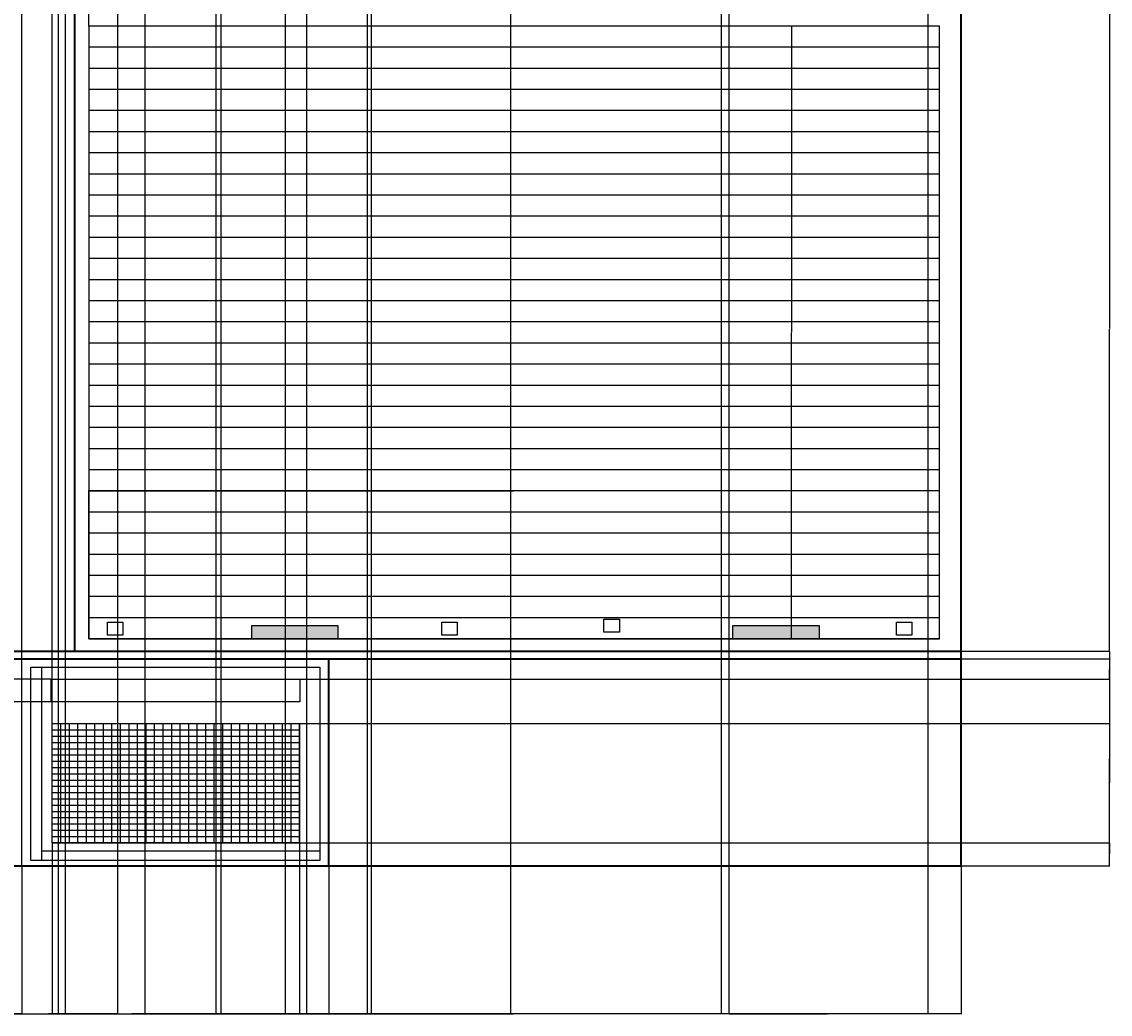
# Model space of a CAD drawing. Units: inches. Extents: x 1231 to 2151, y 481 to 2277.
# Tile 3 of 7: x 1542 to 2151, y 481 to 1035. Entities that reach past the tile are written whole.
import ezdxf

# ---------------------------------------------------------------- set-up
doc = ezdxf.new("R2010")
doc.units = ezdxf.units.IN
doc.header["$MEASUREMENT"] = 0
for name, color, linetype, lineweight in [('A-ANNO-DIMS', 2, 'Continuous', 18), ('A-DOOR', 4, 'Continuous', 25), ('A-ELEV', 7, 'Continuous', 35), ('A-ELEV-PATT', 9, 'Continuous', 13), ('A-GLAZ', 3, 'Continuous', 25)]:
    doc.layers.add(name, color=color, linetype=linetype, lineweight=lineweight)
doc.styles.get("Standard").update_dxf_attribs({"font": 'arial.ttf'})
doc.dimstyles.get("Standard").update_dxf_attribs({"dimtxt": 0.18, "dimasz": 0.18, "dimexe": 0.18, "dimexo": 0.0625, "dimgap": 0.09, "dimtad": 0, "dimtih": 1, "dimtoh": 1, "dimdec": 0, "dimzin": 0, "dimdsep": 46, "dimlunit": 3, "dimtxsty": 'Standard', "dimcen": 0.09, "dimadec": 0, "dimazin": 0, "dimtfac": 1, "dimtdec": 0, "dimtofl": 0, "dimtmove": 0, "dimatfit": 3, "dimfxl": 1, "dimtolj": 1, "dimtzin": 0, "dimarcsym": 0})

# ---------------------------------------------------------------- blocks, each defined once
blk = doc.blocks.new('*D1')
at = {"layer": 'A-ANNO-DIMS', "color": 0, "lineweight": -2, "transparency": 16777216}
for p, q in [((1314.24, 563.63), (1314.24, 480.76)), ((2067.47, 563.63), (2067.47, 480.76)), ((1314.42, 480.94), (1690.47, 480.94)), ((2067.29, 480.94), (1691.25, 480.94))]:
    blk.add_line(p, q, dxfattribs=at)
at = {"layer": 'A-ANNO-DIMS', "color": 0, "transparency": 16777216}
for points in [[(1314.42, 480.97), (1314.42, 480.91), (1314.24, 480.94)], [(2067.29, 480.97), (2067.29, 480.91), (2067.47, 480.94)]]:
    blk.add_solid(points, dxfattribs=at)
at = {"layer": 'Defpoints', "color": 0, "transparency": 16777216}
for p in [(1314.24, 563.69), (2067.47, 563.69), (2067.47, 480.94)]:
    blk.add_point(p, dxfattribs=at)
at = {"layer": 'A-ANNO-DIMS', "color": 0, "transparency": 16777216, "insert": (1690.86, 480.94), "char_height": 0.18, "attachment_point": 5}
blk.add_mtext('\\A1;753.2', dxfattribs=at)
blk = doc.blocks.new('*D3')
at = {"layer": 'A-ANNO-DIMS', "color": 0, "lineweight": -2, "transparency": 16777216}
for p, q in [((2067.75, 683.69), (2150.62, 683.69)), ((2150.44, 683.51), (2150.44, 623.87)), ((2150.44, 563.87), (2150.44, 623.51)), ((2067.54, 563.69), (2150.62, 563.69))]:
    blk.add_line(p, q, dxfattribs=at)
at = {"layer": 'A-ANNO-DIMS', "color": 0, "transparency": 16777216}
for points in [[(2150.41, 683.51), (2150.47, 683.51), (2150.44, 683.69)], [(2150.41, 563.87), (2150.47, 563.87), (2150.44, 563.69)]]:
    blk.add_solid(points, dxfattribs=at)
at = {"layer": 'Defpoints', "color": 0, "transparency": 16777216}
for p in [(2067.69, 683.69), (2150.44, 683.69), (2067.47, 563.69)]:
    blk.add_point(p, dxfattribs=at)
at = {"layer": 'A-ANNO-DIMS', "color": 0, "transparency": 16777216, "insert": (2150.44, 623.69), "char_height": 0.18, "attachment_point": 5}
blk.add_mtext('\\A1;120', dxfattribs=at)
blk = doc.blocks.new('*D4')
at = {"layer": 'A-ANNO-DIMS', "color": 0, "lineweight": -2, "transparency": 16777216}
for p, q in [((2067.75, 1043.69), (2150.62, 1043.69)), ((2150.44, 1043.51), (2150.44, 863.87)), ((2150.44, 683.87), (2150.44, 863.51)), ((2067.75, 683.69), (2150.62, 683.69))]:
    blk.add_line(p, q, dxfattribs=at)
at = {"layer": 'A-ANNO-DIMS', "color": 0, "transparency": 16777216}
for points in [[(2150.41, 1043.51), (2150.47, 1043.51), (2150.44, 1043.69)], [(2150.41, 683.87), (2150.47, 683.87), (2150.44, 683.69)]]:
    blk.add_solid(points, dxfattribs=at)
at = {"layer": 'Defpoints', "color": 0, "transparency": 16777216}
for p in [(2067.69, 1043.69), (2150.44, 1043.69), (2067.69, 683.69)]:
    blk.add_point(p, dxfattribs=at)
at = {"layer": 'A-ANNO-DIMS', "color": 0, "transparency": 16777216, "insert": (2150.44, 863.69), "char_height": 0.18, "attachment_point": 5}
blk.add_mtext('\\A1;360', dxfattribs=at)
blk = doc.blocks.new('*D27')
at = {"layer": 'A-ANNO-DIMS', "color": 0, "lineweight": -2, "transparency": 16777216}
for p, q in [((2055.26, 1032.81), (1972.39, 1032.81)), ((1972.57, 1032.63), (1972.57, 861.82)), ((1972.57, 690.64), (1972.57, 861.45)), ((2055.26, 690.46), (1972.39, 690.46))]:
    blk.add_line(p, q, dxfattribs=at)
at = {"layer": 'A-ANNO-DIMS', "color": 0, "transparency": 16777216}
for points in [[(1972.54, 1032.63), (1972.6, 1032.63), (1972.57, 1032.81)], [(1972.54, 690.64), (1972.6, 690.64), (1972.57, 690.46)]]:
    blk.add_solid(points, dxfattribs=at)
at = {"layer": 'Defpoints', "color": 0, "transparency": 16777216}
for p in [(1972.57, 1032.81), (2055.32, 1032.81), (2055.32, 690.46)]:
    blk.add_point(p, dxfattribs=at)
at = {"layer": 'A-ANNO-DIMS', "color": 0, "transparency": 16777216, "insert": (1972.57, 861.64), "char_height": 0.18, "attachment_point": 5}
blk.add_mtext('\\A1;342.35', dxfattribs=at)
blk = doc.blocks.new('*D28')
at = {"layer": 'A-ANNO-DIMS', "color": 0, "lineweight": -2, "transparency": 16777216}
for p, q in [((1579.79, 690.52), (1579.79, 773.39)), ((1579.97, 773.21), (1817.16, 773.21)), ((2055.14, 773.21), (1817.95, 773.21)), ((2055.32, 690.52), (2055.32, 773.39))]:
    blk.add_line(p, q, dxfattribs=at)
at = {"layer": 'A-ANNO-DIMS', "color": 0, "transparency": 16777216}
for points in [[(1579.97, 773.24), (1579.97, 773.18), (1579.79, 773.21)], [(2055.14, 773.24), (2055.14, 773.18), (2055.32, 773.21)]]:
    blk.add_solid(points, dxfattribs=at)
at = {"layer": 'Defpoints', "color": 0, "transparency": 16777216}
for p in [(2055.32, 773.21), (1579.79, 690.46), (2055.32, 690.46)]:
    blk.add_point(p, dxfattribs=at)
at = {"layer": 'A-ANNO-DIMS', "color": 0, "transparency": 16777216, "insert": (1817.56, 773.21), "char_height": 0.18, "attachment_point": 5}
blk.add_mtext('\\A1;475.5', dxfattribs=at)
blk = doc.blocks.new('*D36')
at = {"layer": 'A-ANNO-DIMS', "color": 0, "lineweight": -2, "transparency": 16777216}
for p, q in [((1571.76, 1043.75), (1571.76, 2276.71)), ((1571.94, 2276.53), (1575.38, 2276.53)), ((1579.61, 2276.53), (1576.17, 2276.53)), ((1579.79, 1032.87), (1579.79, 2276.71))]:
    blk.add_line(p, q, dxfattribs=at)
at = {"layer": 'A-ANNO-DIMS', "color": 0, "transparency": 16777216}
for points in [[(1571.94, 2276.56), (1571.94, 2276.5), (1571.76, 2276.53)], [(1579.61, 2276.56), (1579.61, 2276.5), (1579.79, 2276.53)]]:
    blk.add_solid(points, dxfattribs=at)
at = {"layer": 'Defpoints', "color": 0, "transparency": 16777216}
for p in [(1579.79, 2276.53), (1571.76, 1043.69), (1579.79, 1032.81)]:
    blk.add_point(p, dxfattribs=at)
at = {"layer": 'A-ANNO-DIMS', "color": 0, "transparency": 16777216, "insert": (1575.78, 2276.53), "char_height": 0.18, "attachment_point": 5}
blk.add_mtext('\\A1;8.033', dxfattribs=at)
blk = doc.blocks.new('*D48')
at = {"layer": 'A-ANNO-DIMS', "color": 0, "lineweight": -2, "transparency": 16777216}
for p, q in [((1314.24, 563.63), (1314.24, 480.76)), ((1542.38, 563.63), (1542.38, 480.76)), ((1314.42, 480.94), (1427.84, 480.94)), ((1542.2, 480.94), (1428.77, 480.94))]:
    blk.add_line(p, q, dxfattribs=at)
at = {"layer": 'A-ANNO-DIMS', "color": 0, "transparency": 16777216}
for points in [[(1314.42, 480.97), (1314.42, 480.91), (1314.24, 480.94)], [(1542.2, 480.97), (1542.2, 480.91), (1542.38, 480.94)]]:
    blk.add_solid(points, dxfattribs=at)
at = {"layer": 'Defpoints', "color": 0, "transparency": 16777216}
for p in [(1314.24, 563.69), (1542.38, 563.69), (1542.38, 480.94)]:
    blk.add_point(p, dxfattribs=at)
at = {"layer": 'A-ANNO-DIMS', "color": 0, "transparency": 16777216, "insert": (1428.31, 480.94), "char_height": 0.18, "attachment_point": 5}
blk.add_mtext('\\A1;228.13', dxfattribs=at)
blk = doc.blocks.new('*D49')
at = {"layer": 'A-ANNO-DIMS', "color": 0, "lineweight": -2, "transparency": 16777216}
for p, q in [((1542.38, 563.63), (1542.38, 480.76)), ((1714.02, 563.63), (1714.02, 480.76)), ((1542.56, 480.94), (1627.74, 480.94)), ((1713.84, 480.94), (1628.65, 480.94))]:
    blk.add_line(p, q, dxfattribs=at)
at = {"layer": 'A-ANNO-DIMS', "color": 0, "transparency": 16777216}
for points in [[(1542.56, 480.97), (1542.56, 480.91), (1542.38, 480.94)], [(1713.84, 480.97), (1713.84, 480.91), (1714.02, 480.94)]]:
    blk.add_solid(points, dxfattribs=at)
at = {"layer": 'Defpoints', "color": 0, "transparency": 16777216}
for p in [(1542.38, 563.69), (1714.02, 563.69), (1714.02, 480.94)]:
    blk.add_point(p, dxfattribs=at)
at = {"layer": 'A-ANNO-DIMS', "color": 0, "transparency": 16777216, "insert": (1628.2, 480.94), "char_height": 0.18, "attachment_point": 5}
blk.add_mtext('\\A1;171.65', dxfattribs=at)
blk = doc.blocks.new('*D50')
at = {"layer": 'A-ANNO-DIMS', "color": 0, "lineweight": -2, "transparency": 16777216}
for p, q in [((1542.38, 563.75), (1542.38, 2276.71)), ((1542.56, 2276.53), (1550.52, 2276.53)), ((1559.26, 2276.53), (1551.3, 2276.53)), ((1559.44, 576.65), (1559.44, 2276.71))]:
    blk.add_line(p, q, dxfattribs=at)
at = {"layer": 'A-ANNO-DIMS', "color": 0, "transparency": 16777216}
for points in [[(1542.56, 2276.56), (1542.56, 2276.5), (1542.38, 2276.53)], [(1559.26, 2276.56), (1559.26, 2276.5), (1559.44, 2276.53)]]:
    blk.add_solid(points, dxfattribs=at)
at = {"layer": 'Defpoints', "color": 0, "transparency": 16777216}
for p in [(1559.44, 2276.53), (1559.44, 576.59), (1542.38, 563.69)]:
    blk.add_point(p, dxfattribs=at)
at = {"layer": 'A-ANNO-DIMS', "color": 0, "transparency": 16777216, "insert": (1550.91, 2276.53), "char_height": 0.18, "attachment_point": 5}
blk.add_mtext('\\A1;17.07', dxfattribs=at)
blk = doc.blocks.new('*D51')
at = {"layer": 'A-ANNO-DIMS', "color": 0, "lineweight": -2, "transparency": 16777216}
for p, q in [((1559.44, 576.53), (1559.44, 480.76)), ((1697.66, 576.53), (1697.66, 480.76)), ((1559.62, 480.94), (1628.17, 480.94)), ((1697.48, 480.94), (1628.94, 480.94))]:
    blk.add_line(p, q, dxfattribs=at)
at = {"layer": 'A-ANNO-DIMS', "color": 0, "transparency": 16777216}
for points in [[(1559.62, 480.97), (1559.62, 480.91), (1559.44, 480.94)], [(1697.48, 480.97), (1697.48, 480.91), (1697.66, 480.94)]]:
    blk.add_solid(points, dxfattribs=at)
at = {"layer": 'Defpoints', "color": 0, "transparency": 16777216}
for p in [(1559.44, 576.59), (1697.66, 576.59), (1697.66, 480.94)]:
    blk.add_point(p, dxfattribs=at)
at = {"layer": 'A-ANNO-DIMS', "color": 0, "transparency": 16777216, "insert": (1628.55, 480.94), "char_height": 0.18, "attachment_point": 5}
blk.add_mtext('\\A1;138.2', dxfattribs=at)
blk = doc.blocks.new('*D52')
at = {"layer": 'A-ANNO-DIMS', "color": 0, "lineweight": -2, "transparency": 16777216}
for p, q in [((1697.72, 576.59), (2150.62, 576.59)), ((2150.44, 576.41), (2150.44, 570.32)), ((2150.44, 563.87), (2150.44, 569.96)), ((1714.09, 563.69), (2150.62, 563.69))]:
    blk.add_line(p, q, dxfattribs=at)
at = {"layer": 'A-ANNO-DIMS', "color": 0, "transparency": 16777216}
for points in [[(2150.41, 576.41), (2150.47, 576.41), (2150.44, 576.59)], [(2150.41, 563.87), (2150.47, 563.87), (2150.44, 563.69)]]:
    blk.add_solid(points, dxfattribs=at)
at = {"layer": 'Defpoints', "color": 0, "transparency": 16777216}
for p in [(1697.66, 576.59), (2150.44, 576.59), (1714.02, 563.69)]:
    blk.add_point(p, dxfattribs=at)
at = {"layer": 'A-ANNO-DIMS', "color": 0, "transparency": 16777216, "insert": (2150.44, 570.14), "char_height": 0.18, "attachment_point": 5}
blk.add_mtext('\\A1;12.898', dxfattribs=at)
blk = doc.blocks.new('*D53')
at = {"layer": 'A-ANNO-DIMS', "color": 0, "lineweight": -2, "transparency": 16777216}
for p, q in [((1697.72, 643.11), (2150.62, 643.11)), ((2150.44, 642.93), (2150.44, 610.03)), ((2150.44, 576.77), (2150.44, 609.67)), ((1697.72, 576.59), (2150.62, 576.59))]:
    blk.add_line(p, q, dxfattribs=at)
at = {"layer": 'A-ANNO-DIMS', "color": 0, "transparency": 16777216}
for points in [[(2150.41, 642.93), (2150.47, 642.93), (2150.44, 643.11)], [(2150.41, 576.77), (2150.47, 576.77), (2150.44, 576.59)]]:
    blk.add_solid(points, dxfattribs=at)
at = {"layer": 'Defpoints', "color": 0, "transparency": 16777216}
for p in [(1697.66, 643.11), (2150.44, 643.11), (1697.66, 576.59)]:
    blk.add_point(p, dxfattribs=at)
at = {"layer": 'A-ANNO-DIMS', "color": 0, "transparency": 16777216, "insert": (2150.44, 609.85), "char_height": 0.18, "attachment_point": 5}
blk.add_mtext('\\A1;66.52', dxfattribs=at)
blk = doc.blocks.new('*D54')
at = {"layer": 'A-ANNO-DIMS', "color": 0, "lineweight": -2, "transparency": 16777216}
for p, q in [((1714.09, 679.24), (2150.62, 679.24)), ((2150.44, 679.06), (2150.44, 673.81)), ((2150.44, 668.2), (2150.44, 673.45)), ((1697.86, 668.02), (2150.62, 668.02))]:
    blk.add_line(p, q, dxfattribs=at)
at = {"layer": 'A-ANNO-DIMS', "color": 0, "transparency": 16777216}
for points in [[(2150.41, 679.06), (2150.47, 679.06), (2150.44, 679.24)], [(2150.41, 668.2), (2150.47, 668.2), (2150.44, 668.02)]]:
    blk.add_solid(points, dxfattribs=at)
at = {"layer": 'Defpoints', "color": 0, "transparency": 16777216}
for p in [(1714.02, 679.24), (2150.44, 679.24), (1697.8, 668.02)]:
    blk.add_point(p, dxfattribs=at)
at = {"layer": 'A-ANNO-DIMS', "color": 0, "transparency": 16777216, "insert": (2150.44, 673.63), "char_height": 0.18, "attachment_point": 5}
blk.add_mtext('\\A1;11.222', dxfattribs=at)
blk = doc.blocks.new('*D55')
at = {"layer": 'A-ANNO-DIMS', "color": 0, "lineweight": -2, "transparency": 16777216}
for p, q in [((1558.65, 668.02), (1230.78, 668.02)), ((1230.96, 667.84), (1230.96, 661.8)), ((1230.96, 655.39), (1230.96, 661.43)), ((1558.65, 655.21), (1230.78, 655.21))]:
    blk.add_line(p, q, dxfattribs=at)
at = {"layer": 'A-ANNO-DIMS', "color": 0, "transparency": 16777216}
for points in [[(1230.93, 667.84), (1230.99, 667.84), (1230.96, 668.02)], [(1230.93, 655.39), (1230.99, 655.39), (1230.96, 655.21)]]:
    blk.add_solid(points, dxfattribs=at)
at = {"layer": 'Defpoints', "color": 0, "transparency": 16777216}
for p in [(1230.96, 668.02), (1558.72, 668.02), (1558.72, 655.21)]:
    blk.add_point(p, dxfattribs=at)
at = {"layer": 'A-ANNO-DIMS', "color": 0, "transparency": 16777216, "insert": (1230.96, 661.62), "char_height": 0.18, "attachment_point": 5}
blk.add_mtext('\\A1;12.808', dxfattribs=at)
blk = doc.blocks.new('*D56')
at = {"layer": 'A-ANNO-DIMS', "color": 0, "lineweight": -2, "transparency": 16777216}
for p, q in [((1714.09, 679.24), (2150.62, 679.24)), ((2150.44, 679.06), (2150.44, 621.65)), ((2150.44, 563.87), (2150.44, 621.29)), ((1714.09, 563.69), (2150.62, 563.69))]:
    blk.add_line(p, q, dxfattribs=at)
at = {"layer": 'A-ANNO-DIMS', "color": 0, "transparency": 16777216}
for points in [[(2150.41, 679.06), (2150.47, 679.06), (2150.44, 679.24)], [(2150.41, 563.87), (2150.47, 563.87), (2150.44, 563.69)]]:
    blk.add_solid(points, dxfattribs=at)
at = {"layer": 'Defpoints', "color": 0, "transparency": 16777216}
for p in [(1714.02, 679.24), (2150.44, 679.24), (1714.02, 563.69)]:
    blk.add_point(p, dxfattribs=at)
at = {"layer": 'A-ANNO-DIMS', "color": 0, "transparency": 16777216, "insert": (2150.44, 621.47), "char_height": 0.18, "attachment_point": 5}
blk.add_mtext('\\A1;115.55', dxfattribs=at)
blk = doc.blocks.new('*D69')
at = {"layer": 'A-ANNO-DIMS', "color": 0, "lineweight": -2, "transparency": 16777216}
for p, q in [((1512.01, 1085.65), (1512.01, 480.76)), ((1937.57, 1085.65), (1937.57, 480.76)), ((1512.19, 480.94), (1724.39, 480.94)), ((1937.39, 480.94), (1725.19, 480.94))]:
    blk.add_line(p, q, dxfattribs=at)
at = {"layer": 'A-ANNO-DIMS', "color": 0, "transparency": 16777216}
for points in [[(1512.19, 480.97), (1512.19, 480.91), (1512.01, 480.94)], [(1937.39, 480.97), (1937.39, 480.91), (1937.57, 480.94)]]:
    blk.add_solid(points, dxfattribs=at)
at = {"layer": 'Defpoints', "color": 0, "transparency": 16777216}
for p in [(1512.01, 1085.71), (1937.57, 1085.71), (1937.57, 480.94)]:
    blk.add_point(p, dxfattribs=at)
at = {"layer": 'A-ANNO-DIMS', "color": 0, "transparency": 16777216, "insert": (1724.79, 480.94), "char_height": 0.18, "attachment_point": 5}
blk.add_mtext('\\A1;425.6', dxfattribs=at)
blk = doc.blocks.new('*D71')
at = {"layer": 'A-ANNO-DIMS', "color": 0, "lineweight": -2, "transparency": 16777216}
for p, q in [((1517.5, 1116.1), (1517.5, 480.76)), ((1595.89, 1116.1), (1595.89, 480.76)), ((1517.68, 480.94), (1556.31, 480.94)), ((1595.71, 480.94), (1557.09, 480.94))]:
    blk.add_line(p, q, dxfattribs=at)
at = {"layer": 'A-ANNO-DIMS', "color": 0, "transparency": 16777216}
for points in [[(1517.68, 480.97), (1517.68, 480.91), (1517.5, 480.94)], [(1595.71, 480.97), (1595.71, 480.91), (1595.89, 480.94)]]:
    blk.add_solid(points, dxfattribs=at)
at = {"layer": 'Defpoints', "color": 0, "transparency": 16777216}
for p in [(1517.5, 1116.16), (1595.89, 1116.16), (1595.89, 480.94)]:
    blk.add_point(p, dxfattribs=at)
at = {"layer": 'A-ANNO-DIMS', "color": 0, "transparency": 16777216, "insert": (1556.7, 480.94), "char_height": 0.18, "attachment_point": 5}
blk.add_mtext('\\A1;78.39', dxfattribs=at)
blk = doc.blocks.new('*D72')
at = {"layer": 'A-ANNO-DIMS', "color": 0, "lineweight": -2, "transparency": 16777216}
for p, q in [((1595.89, 1116.1), (1595.89, 480.76)), ((1611.14, 1116.1), (1611.14, 480.76)), ((1596.07, 480.94), (1603.13, 480.94)), ((1610.96, 480.94), (1603.9, 480.94))]:
    blk.add_line(p, q, dxfattribs=at)
at = {"layer": 'A-ANNO-DIMS', "color": 0, "transparency": 16777216}
for points in [[(1596.07, 480.97), (1596.07, 480.91), (1595.89, 480.94)], [(1610.96, 480.97), (1610.96, 480.91), (1611.14, 480.94)]]:
    blk.add_solid(points, dxfattribs=at)
at = {"layer": 'Defpoints', "color": 0, "transparency": 16777216}
for p in [(1595.89, 1116.16), (1611.14, 1116.16), (1611.14, 480.94)]:
    blk.add_point(p, dxfattribs=at)
at = {"layer": 'A-ANNO-DIMS', "color": 0, "transparency": 16777216, "insert": (1603.52, 480.94), "char_height": 0.18, "attachment_point": 5}
blk.add_mtext('\\A1;15.25', dxfattribs=at)
blk = doc.blocks.new('*D73')
at = {"layer": 'A-ANNO-DIMS', "color": 0, "lineweight": -2, "transparency": 16777216}
for p, q in [((1611.14, 1116.1), (1611.14, 480.76)), ((1689.53, 1116.1), (1689.53, 480.76)), ((1611.32, 480.94), (1649.94, 480.94)), ((1689.35, 480.94), (1650.73, 480.94))]:
    blk.add_line(p, q, dxfattribs=at)
at = {"layer": 'A-ANNO-DIMS', "color": 0, "transparency": 16777216}
for points in [[(1611.32, 480.97), (1611.32, 480.91), (1611.14, 480.94)], [(1689.35, 480.97), (1689.35, 480.91), (1689.53, 480.94)]]:
    blk.add_solid(points, dxfattribs=at)
at = {"layer": 'Defpoints', "color": 0, "transparency": 16777216}
for p in [(1611.14, 1116.16), (1689.53, 1116.16), (1689.53, 480.94)]:
    blk.add_point(p, dxfattribs=at)
at = {"layer": 'A-ANNO-DIMS', "color": 0, "transparency": 16777216, "insert": (1650.34, 480.94), "char_height": 0.18, "attachment_point": 5}
blk.add_mtext('\\A1;78.39', dxfattribs=at)
blk = doc.blocks.new('*D74')
at = {"layer": 'A-ANNO-DIMS', "color": 0, "lineweight": -2, "transparency": 16777216}
for p, q in [((1689.53, 1116.1), (1689.53, 480.76)), ((1701.52, 1116.1), (1701.52, 480.76)), ((1689.71, 480.94), (1695.07, 480.94)), ((1701.34, 480.94), (1695.98, 480.94))]:
    blk.add_line(p, q, dxfattribs=at)
at = {"layer": 'A-ANNO-DIMS', "color": 0, "transparency": 16777216}
for points in [[(1689.71, 480.97), (1689.71, 480.91), (1689.53, 480.94)], [(1701.34, 480.97), (1701.34, 480.91), (1701.52, 480.94)]]:
    blk.add_solid(points, dxfattribs=at)
at = {"layer": 'Defpoints', "color": 0, "transparency": 16777216}
for p in [(1689.53, 1116.16), (1701.52, 1116.16), (1701.52, 480.94)]:
    blk.add_point(p, dxfattribs=at)
at = {"layer": 'A-ANNO-DIMS', "color": 0, "transparency": 16777216, "insert": (1695.53, 480.94), "char_height": 0.18, "attachment_point": 5}
blk.add_mtext('\\A1;11.992', dxfattribs=at)
blk = doc.blocks.new('*D75')
at = {"layer": 'A-ANNO-DIMS', "color": 0, "lineweight": -2, "transparency": 16777216}
for p, q in [((1701.52, 1116.1), (1701.52, 480.76)), ((1933.36, 1116.1), (1933.36, 480.76)), ((1701.7, 480.94), (1816.97, 480.94)), ((1933.18, 480.94), (1817.9, 480.94))]:
    blk.add_line(p, q, dxfattribs=at)
at = {"layer": 'A-ANNO-DIMS', "color": 0, "transparency": 16777216}
for points in [[(1701.7, 480.97), (1701.7, 480.91), (1701.52, 480.94)], [(1933.18, 480.97), (1933.18, 480.91), (1933.36, 480.94)]]:
    blk.add_solid(points, dxfattribs=at)
at = {"layer": 'Defpoints', "color": 0, "transparency": 16777216}
for p in [(1701.52, 1116.16), (1933.36, 1116.16), (1933.36, 480.94)]:
    blk.add_point(p, dxfattribs=at)
at = {"layer": 'A-ANNO-DIMS', "color": 0, "transparency": 16777216, "insert": (1817.44, 480.94), "char_height": 0.18, "attachment_point": 5}
blk.add_mtext('\\A1;231.83', dxfattribs=at)
blk = doc.blocks.new('*D80')
at = {"layer": 'A-ANNO-DIMS', "color": 0, "lineweight": -2, "transparency": 16777216}
for p, q in [((1937.57, 1170.27), (1937.57, 480.76)), ((2048.89, 1126.2), (2048.89, 480.76)), ((1937.75, 480.94), (1992.79, 480.94)), ((2048.71, 480.94), (1993.67, 480.94))]:
    blk.add_line(p, q, dxfattribs=at)
at = {"layer": 'A-ANNO-DIMS', "color": 0, "transparency": 16777216}
for points in [[(1937.75, 480.97), (1937.75, 480.91), (1937.57, 480.94)], [(2048.71, 480.97), (2048.71, 480.91), (2048.89, 480.94)]]:
    blk.add_solid(points, dxfattribs=at)
at = {"layer": 'Defpoints', "color": 0, "transparency": 16777216}
for p in [(1937.57, 1170.34), (2048.89, 1126.26), (2048.89, 480.94)]:
    blk.add_point(p, dxfattribs=at)
at = {"layer": 'A-ANNO-DIMS', "color": 0, "transparency": 16777216, "insert": (1993.23, 480.94), "char_height": 0.18, "attachment_point": 5}
blk.add_mtext('\\A1;111.31', dxfattribs=at)
blk = doc.blocks.new('*D90')
at = {"layer": 'A-ANNO-DIMS', "color": 0, "lineweight": -2, "transparency": 16777216}
for p, q in [((1566.56, 1479.25), (1566.56, 480.76)), ((1562.79, 1475.48), (1562.79, 480.76)), ((1562.97, 480.94), (1564.3, 480.94)), ((1566.38, 480.94), (1565.05, 480.94))]:
    blk.add_line(p, q, dxfattribs=at)
at = {"layer": 'A-ANNO-DIMS', "color": 0, "transparency": 16777216}
for points in [[(1562.97, 480.97), (1562.97, 480.91), (1562.79, 480.94)], [(1566.38, 480.97), (1566.38, 480.91), (1566.56, 480.94)]]:
    blk.add_solid(points, dxfattribs=at)
at = {"layer": 'Defpoints', "color": 0, "transparency": 16777216}
for p in [(1566.56, 1479.32), (1562.79, 1475.54), (1566.56, 480.94)]:
    blk.add_point(p, dxfattribs=at)
at = {"layer": 'A-ANNO-DIMS', "color": 0, "transparency": 16777216, "insert": (1564.68, 480.94), "char_height": 0.18, "attachment_point": 5}
blk.add_mtext('\\A1;3.771', dxfattribs=at)
blk = doc.blocks.new('*D91')
at = {"layer": 'A-ANNO-DIMS', "color": 0, "lineweight": -2, "transparency": 16777216}
for p, q in [((1566.56, 1479.25), (1566.56, 480.76)), ((1650.77, 1479.25), (1650.77, 480.76)), ((1566.74, 480.94), (1608.34, 480.94)), ((1650.59, 480.94), (1608.99, 480.94))]:
    blk.add_line(p, q, dxfattribs=at)
at = {"layer": 'A-ANNO-DIMS', "color": 0, "transparency": 16777216}
for points in [[(1566.74, 480.97), (1566.74, 480.91), (1566.56, 480.94)], [(1650.59, 480.97), (1650.59, 480.91), (1650.77, 480.94)]]:
    blk.add_solid(points, dxfattribs=at)
at = {"layer": 'Defpoints', "color": 0, "transparency": 16777216}
for p in [(1566.56, 1479.32), (1650.77, 1479.32), (1650.77, 480.94)]:
    blk.add_point(p, dxfattribs=at)
at = {"layer": 'A-ANNO-DIMS', "color": 0, "transparency": 16777216, "insert": (1608.66, 480.94), "char_height": 0.18, "attachment_point": 5}
blk.add_mtext('\\A1;84.2', dxfattribs=at)
blk = doc.blocks.new('*D92')
at = {"layer": 'A-ANNO-DIMS', "color": 0, "lineweight": -2, "transparency": 16777216}
for p, q in [((1653.67, 1479.25), (1653.67, 480.76)), ((1735.42, 1479.25), (1735.42, 480.76)), ((1653.85, 480.94), (1694.15, 480.94)), ((1735.24, 480.94), (1694.94, 480.94))]:
    blk.add_line(p, q, dxfattribs=at)
at = {"layer": 'A-ANNO-DIMS', "color": 0, "transparency": 16777216}
for points in [[(1653.85, 480.97), (1653.85, 480.91), (1653.67, 480.94)], [(1735.24, 480.97), (1735.24, 480.91), (1735.42, 480.94)]]:
    blk.add_solid(points, dxfattribs=at)
at = {"layer": 'Defpoints', "color": 0, "transparency": 16777216}
for p in [(1653.67, 1479.32), (1735.42, 1479.32), (1735.42, 480.94)]:
    blk.add_point(p, dxfattribs=at)
at = {"layer": 'A-ANNO-DIMS', "color": 0, "transparency": 16777216, "insert": (1694.55, 480.94), "char_height": 0.18, "attachment_point": 5}
blk.add_mtext('\\A1;81.75', dxfattribs=at)
blk = doc.blocks.new('*D93')
at = {"layer": 'A-ANNO-DIMS', "color": 0, "lineweight": -2, "transparency": 16777216}
for p, q in [((1737.75, 1479.25), (1737.75, 480.76)), ((1815.54, 1479.25), (1815.54, 480.76)), ((1737.93, 480.94), (1776.25, 480.94)), ((1815.36, 480.94), (1777.04, 480.94))]:
    blk.add_line(p, q, dxfattribs=at)
at = {"layer": 'A-ANNO-DIMS', "color": 0, "transparency": 16777216}
for points in [[(1737.93, 480.97), (1737.93, 480.91), (1737.75, 480.94)], [(1815.36, 480.97), (1815.36, 480.91), (1815.54, 480.94)]]:
    blk.add_solid(points, dxfattribs=at)
at = {"layer": 'Defpoints', "color": 0, "transparency": 16777216}
for p in [(1737.75, 1479.32), (1815.54, 1479.32), (1815.54, 480.94)]:
    blk.add_point(p, dxfattribs=at)
at = {"layer": 'A-ANNO-DIMS', "color": 0, "transparency": 16777216, "insert": (1776.64, 480.94), "char_height": 0.18, "attachment_point": 5}
blk.add_mtext('\\A1;77.79', dxfattribs=at)

msp = doc.modelspace()

# ---------------------------------------------------------------- hatches: boundary and pattern name
at = {"layer": 'A-ELEV-PATT'}
h = msp.add_hatch(color=256, dxfattribs=at)
h.dxf.hatch_style = 1
h.paths.add_polyline_path([(1719.3246, 697.8114), (1670.7359, 697.8114), (1670.7359, 690.4611), (1719.3246, 690.4611)])
h.paths.add_polyline_path([(1988.2874, 697.8114), (1939.6987, 697.8114), (1939.6987, 690.4611), (1988.2874, 690.4611)])

# ---------------------------------------------------------------- linework, layer by layer
at = {"layer": 'A-DOOR'}
for p, q in [((2055.3191, 1032.8111), (1579.7928, 1032.8111)), ((1579.7928, 1032.8111), (1579.7928, 690.4611)), ((2055.3191, 690.4611), (2055.3191, 1032.8111)), ((2055.3191, 1021.006), (1579.7928, 1021.006)), ((2055.3191, 1009.2008), (1579.7928, 1009.2008)), ((2055.3191, 997.3956), (1579.7928, 997.3956)), ((2055.3191, 985.5904), (1579.7928, 985.5904)), ((2055.3191, 973.7853), (1579.7928, 973.7853)), ((2055.3191, 961.9801), (1579.7928, 961.9801)), ((2055.3191, 950.1749), (1579.7928, 950.1749)), ((2055.3191, 938.3697), (1579.7928, 938.3697)), ((2055.3191, 926.5646), (1579.7928, 926.5646)), ((2055.3191, 914.7594), (1579.7928, 914.7594)), ((2055.3191, 902.9542), (1579.7928, 902.9542)), ((2055.3191, 891.1491), (1579.7928, 891.1491)), ((2055.3191, 879.3439), (1579.7928, 879.3439)), ((2055.3191, 867.5387), (1579.7928, 867.5387)), ((2055.3191, 855.7335), (1579.7928, 855.7335)), ((2055.3191, 843.9284), (1579.7928, 843.9284)), ((2055.3191, 832.1232), (1579.7928, 832.1232)), ((2055.3191, 820.318), (1579.7928, 820.318)), ((2055.3191, 808.5129), (1579.7928, 808.5129)), ((2055.3191, 796.7077), (1579.7928, 796.7077)), ((2055.3191, 784.9025), (1579.7928, 784.9025)), ((2055.3191, 773.0973), (1579.7928, 773.0973)), ((2055.3191, 761.2922), (1579.7928, 761.2922)), ((2055.3191, 749.487), (1579.7928, 749.487)), ((2055.3191, 737.6818), (1579.7928, 737.6818)), ((2055.3191, 725.8766), (1579.7928, 725.8766)), ((2055.3191, 714.0715), (1579.7928, 714.0715)), ((2055.3191, 702.2663), (1579.7928, 702.2663)), ((1579.7928, 690.4611), (2055.3191, 690.4611)), ((2055.3191, 690.4611), (1579.7928, 690.4611))]:
    msp.add_line(p, q, dxfattribs=at)
for points in [[(1590.3593, 699.8327), (1598.9581, 699.8327), (1598.9581, 692.4836), (1590.3593, 692.4836)], [(1777.1541, 699.8327), (1785.7529, 699.8327), (1785.7529, 692.4836), (1777.1541, 692.4836)], [(1867.8069, 701.4848), (1876.4058, 701.4848), (1876.4058, 694.1357), (1867.8069, 694.1357)], [(2031.3087, 699.8327), (2039.9075, 699.8327), (2039.9075, 692.4836), (2031.3087, 692.4836)], [(1670.7359, 690.4611), (1719.3246, 690.4611), (1719.3246, 697.8114), (1670.7359, 697.8114)], [(1939.6987, 690.4611), (1988.2874, 690.4611), (1988.2874, 697.8114), (1939.6987, 697.8114)]]:
    msp.add_lwpolyline(points, close=True, dxfattribs=at)
at = {"layer": 'A-ELEV'}
for p, q in [((2067.4747, 563.6912), (2067.4747, 2193.7789)), ((1571.76, 1043.6912), (1571.76, 683.6912)), ((1314.2408, 683.6912), (2067.6855, 683.6912)), ((1313.7129, 679.2431), (2067.6855, 679.2431)), ((1313.7129, 679.2431), (2067.6855, 679.2431)), ((1714.0227, 563.6912), (1714.0227, 679.2431)), ((1314.2408, 563.6912), (2067.6855, 563.6912))]:
    msp.add_line(p, q, dxfattribs=at)
at = {"layer": 'A-GLAZ'}
for p, q in [((1547.4014, 674.6113), (1708.9402, 674.6113)), ((1547.4014, 566.5596), (1547.4014, 674.6113)), ((1553.5797, 566.5596), (1553.5797, 674.6113)), ((1708.9402, 674.6113), (1708.9402, 566.5596)), ((1559.4446, 643.1096), (1697.6571, 643.1096)), ((1559.4446, 576.5889), (1559.4446, 643.1096)), ((1559.4446, 639.6085), (1697.6571, 639.6085)), ((1564.2106, 576.5889), (1564.2106, 643.1096)), ((1568.9765, 576.5889), (1568.9765, 643.1096)), ((1573.7425, 576.5889), (1573.7425, 643.1096)), ((1578.5084, 576.5889), (1578.5084, 643.1096)), ((1583.2744, 576.5889), (1583.2744, 643.1096)), ((1588.0403, 576.5889), (1588.0403, 643.1096)), ((1592.8063, 576.5889), (1592.8063, 643.1096)), ((1597.5722, 576.5889), (1597.5722, 643.1096)), ((1602.3382, 576.5889), (1602.3382, 643.1096)), ((1607.1041, 576.5889), (1607.1041, 643.1096)), ((1611.8701, 576.5889), (1611.8701, 643.1096)), ((1616.636, 576.5889), (1616.636, 643.1096)), ((1621.402, 576.5889), (1621.402, 643.1096)), ((1626.1679, 576.5889), (1626.1679, 643.1096)), ((1630.9339, 576.5889), (1630.9339, 643.1096)), ((1635.6998, 576.5889), (1635.6998, 643.1096)), ((1640.4658, 576.5889), (1640.4658, 643.1096)), ((1645.2317, 576.5889), (1645.2317, 643.1096)), ((1649.9977, 576.5889), (1649.9977, 643.1096)), ((1654.7636, 576.5889), (1654.7636, 643.1096)), ((1659.5296, 576.5889), (1659.5296, 643.1096)), ((1664.2955, 576.5889), (1664.2955, 643.1096)), ((1669.0614, 576.5889), (1669.0614, 643.1096)), ((1673.8274, 576.5889), (1673.8274, 643.1096)), ((1678.5933, 576.5889), (1678.5933, 643.1096)), ((1683.3593, 576.5889), (1683.3593, 643.1096)), ((1688.1252, 576.5889), (1688.1252, 643.1096)), ((1692.8912, 576.5889), (1692.8912, 643.1096)), ((1697.6571, 643.1096), (1697.6571, 576.5889)), ((1697.6571, 576.5889), (1697.6571, 643.1096)), ((1559.4446, 636.1075), (1697.6571, 636.1075)), ((1559.4446, 632.6064), (1697.6571, 632.6064)), ((1559.4446, 629.1053), (1697.6571, 629.1053)), ((1559.4446, 625.6042), (1697.6571, 625.6042)), ((1559.4446, 622.1031), (1697.6571, 622.1031)), ((1559.4446, 618.602), (1697.6571, 618.602)), ((1559.4446, 615.1009), (1697.6571, 615.1009)), ((1559.4446, 611.5998), (1697.6571, 611.5998)), ((1559.4446, 608.0987), (1697.6571, 608.0987)), ((1559.4446, 604.5976), (1697.6571, 604.5976)), ((1559.4446, 601.0965), (1697.6571, 601.0965)), ((1559.4446, 597.5954), (1697.6571, 597.5954)), ((1559.4446, 594.0943), (1697.6571, 594.0943)), ((1559.4446, 590.5933), (1697.6571, 590.5933)), ((1559.4446, 587.0922), (1697.6571, 587.0922)), ((1559.4446, 583.5911), (1697.6571, 583.5911)), ((1559.4446, 580.09), (1697.6571, 580.09)), ((1697.6571, 576.5889), (1559.4446, 576.5889)), ((1559.4446, 576.5889), (1697.6571, 576.5889)), ((1708.9402, 566.5596), (1547.4014, 566.5596)), ((1708.9402, 571.8173), (1553.5797, 571.8173))]:
    msp.add_line(p, q, dxfattribs=at)
msp.add_lwpolyline([(1558.7166, 668.0208), (1697.799, 668.0208), (1697.799, 655.2124), (1558.7166, 655.2124)], close=True, dxfattribs=at)

# ---------------------------------------------------------------- dimensions: what is measured, and where the dimension line sits
at = {"layer": 'A-ANNO-DIMS'}
for base, p1, p2, override, picture, middle in [((1559.4446, 2276.5289), (1542.3752, 563.6912), (1559.4446, 576.5889), {"dimdec": 2, "dimlfac": 1, "dimrnd": 0, "dimzin": 0, "dimdsep": 46, "dimlunit": 2}, '*D50', (1550.9099, 2276.5289)), ((1579.7928, 2276.5289), (1571.76, 1043.6912), (1579.7928, 1032.8111), {"dimdec": 3, "dimlfac": 1, "dimrnd": 0, "dimzin": 0, "dimdsep": 46, "dimlunit": 2}, '*D36', (1575.7764, 2276.5289)), ((1566.5626, 480.9412), (1562.7916, 1475.5441), (1566.5626, 1479.3152), {"dimdec": 3, "dimlfac": 1, "dimrnd": 0, "dimzin": 0, "dimdsep": 46, "dimlunit": 2}, '*D90', (1564.6771, 480.9412)), ((1650.766, 480.9412), (1566.5626, 1479.3152), (1650.766, 1479.3152), {"dimdec": 1, "dimlfac": 1, "dimrnd": 0, "dimzin": 0, "dimdsep": 46, "dimlunit": 2}, '*D91', (1608.6643, 480.9412)), ((1735.4237, 480.9412), (1653.6719, 1479.3152), (1735.4237, 1479.3152), {"dimdec": 2, "dimlfac": 1, "dimrnd": 0, "dimzin": 0, "dimdsep": 46, "dimlunit": 2}, '*D92', (1694.5478, 480.9412)), ((1815.5376, 480.9412), (1737.7463, 1479.3152), (1815.5376, 1479.3152), {"dimdec": 2, "dimlfac": 1, "dimrnd": 0, "dimzin": 0, "dimdsep": 46, "dimlunit": 2}, '*D93', (1776.642, 480.9412)), ((2048.8868, 480.9412), (1937.5725, 1170.3352), (2048.8868, 1126.2615), {"dimdec": 2, "dimlfac": 1, "dimrnd": 0, "dimzin": 0, "dimdsep": 46, "dimlunit": 2}, '*D80', (1993.2297, 480.9412)), ((1595.8928, 480.9412), (1517.5039, 1116.1584), (1595.8928, 1116.1584), {"dimdec": 2, "dimlfac": 1, "dimrnd": 0, "dimzin": 0, "dimdsep": 46, "dimlunit": 2}, '*D71', (1556.6984, 480.9412)), ((1611.1414, 480.9412), (1595.8928, 1116.1584), (1611.1414, 1116.1584), {"dimdec": 2, "dimlfac": 1, "dimrnd": 0, "dimzin": 0, "dimdsep": 46, "dimlunit": 2}, '*D72', (1603.5171, 480.9412)), ((1689.5303, 480.9412), (1611.1414, 1116.1584), (1689.5303, 1116.1584), {"dimdec": 2, "dimlfac": 1, "dimrnd": 0, "dimzin": 0, "dimdsep": 46, "dimlunit": 2}, '*D73', (1650.3359, 480.9412)), ((1701.522, 480.9412), (1689.5303, 1116.1584), (1701.522, 1116.1584), {"dimdec": 3, "dimlfac": 1, "dimrnd": 0, "dimzin": 0, "dimdsep": 46, "dimlunit": 2}, '*D74', (1695.5261, 480.9412)), ((1933.3556, 480.9412), (1701.522, 1116.1584), (1933.3556, 1116.1584), {"dimdec": 2, "dimlfac": 1, "dimrnd": 0, "dimzin": 0, "dimdsep": 46, "dimlunit": 2}, '*D75', (1817.4388, 480.9412)), ((1937.5725, 480.9412), (1512.0105, 1085.7079), (1937.5725, 1085.7079), {"dimdec": 1, "dimlfac": 1, "dimrnd": 0, "dimzin": 0, "dimdsep": 46, "dimlunit": 2}, '*D69', (1724.7915, 480.9412)), ((2055.3191, 773.2111), (1579.7928, 690.4611), (2055.3191, 690.4611), {"dimdec": 1, "dimlfac": 1, "dimrnd": 0, "dimzin": 0, "dimdsep": 46, "dimlunit": 2}, '*D28', (1817.556, 773.2111)), ((1697.6571, 480.9412), (1559.4446, 576.5889), (1697.6571, 576.5889), {"dimdec": 1, "dimlfac": 1, "dimrnd": 0, "dimzin": 0, "dimdsep": 46, "dimlunit": 2}, '*D51', (1628.5509, 480.9412)), ((2067.4747, 480.9412), (1314.2408, 563.6912), (2067.4747, 563.6912), {"dimdec": 1, "dimlfac": 1, "dimrnd": 0, "dimzin": 0, "dimdsep": 46, "dimlunit": 2}, '*D1', (1690.8578, 480.9412)), ((1542.3752, 480.9412), (1314.2408, 563.6912), (1542.3752, 563.6912), {"dimdec": 2, "dimlfac": 1, "dimrnd": 0, "dimzin": 0, "dimdsep": 46, "dimlunit": 2}, '*D48', (1428.308, 480.9412)), ((1714.0227, 480.9412), (1542.3752, 563.6912), (1714.0227, 563.6912), {"dimdec": 2, "dimlfac": 1, "dimrnd": 0, "dimzin": 0, "dimdsep": 46, "dimlunit": 2}, '*D49', (1628.1989, 480.9412))]:
    dim = msp.add_linear_dim(base=base, p1=p1, p2=p2, dimstyle='Standard', override=override, dxfattribs=at)
    dim.commit()
    dim.dimension.update_dxf_attribs({"geometry": picture, "text_midpoint": middle})
for base, p1, p2, override, picture, middle in [((2150.4355, 1043.6912), (2067.6855, 683.6912), (2067.6855, 1043.6912), {"dimdec": 0, "dimlfac": 1, "dimrnd": 0, "dimzin": 0, "dimdsep": 46, "dimlunit": 2}, '*D4', (2150.4355, 863.6912)), ((1972.5691, 1032.8111), (2055.3191, 690.4611), (2055.3191, 1032.8111), {"dimdec": 2, "dimlfac": 1, "dimrnd": 0, "dimzin": 0, "dimdsep": 46, "dimlunit": 2}, '*D27', (1972.5691, 861.6361)), ((2150.4355, 683.6912), (2067.4747, 563.6912), (2067.6855, 683.6912), {"dimdec": 0, "dimlfac": 1, "dimrnd": 0, "dimzin": 0, "dimdsep": 46, "dimlunit": 2}, '*D3', (2150.4355, 623.6912)), ((2150.4355, 679.2431), (1697.799, 668.0208), (1714.0227, 679.2431), {"dimdec": 3, "dimlfac": 1, "dimrnd": 0, "dimzin": 0, "dimdsep": 46, "dimlunit": 2}, '*D54', (2150.4355, 673.632)), ((2150.4355, 679.2431), (1714.0227, 563.6912), (1714.0227, 679.2431), {"dimdec": 2, "dimlfac": 1, "dimrnd": 0, "dimzin": 0, "dimdsep": 46, "dimlunit": 2}, '*D56', (2150.4355, 621.4672)), ((1230.9629, 668.0208), (1558.7166, 655.2124), (1558.7166, 668.0208), {"dimdec": 3, "dimlfac": 1, "dimrnd": 0, "dimzin": 0, "dimdsep": 46, "dimlunit": 2}, '*D55', (1230.9629, 661.6166)), ((2150.4355, 643.1096), (1697.6571, 576.5889), (1697.6571, 643.1096), {"dimdec": 2, "dimlfac": 1, "dimrnd": 0, "dimzin": 0, "dimdsep": 46, "dimlunit": 2}, '*D53', (2150.4355, 609.8493)), ((2150.4355, 576.5889), (1714.0227, 563.6912), (1697.6571, 576.5889), {"dimdec": 3, "dimlfac": 1, "dimrnd": 0, "dimzin": 0, "dimdsep": 46, "dimlunit": 2}, '*D52', (2150.4355, 570.1401))]:
    dim = msp.add_linear_dim(base=base, p1=p1, p2=p2, angle=90, dimstyle='Standard', override=override, dxfattribs=at)
    dim.commit()
    dim.dimension.update_dxf_attribs({"geometry": picture, "text_midpoint": middle})

doc.saveas('drawing.dxf')
